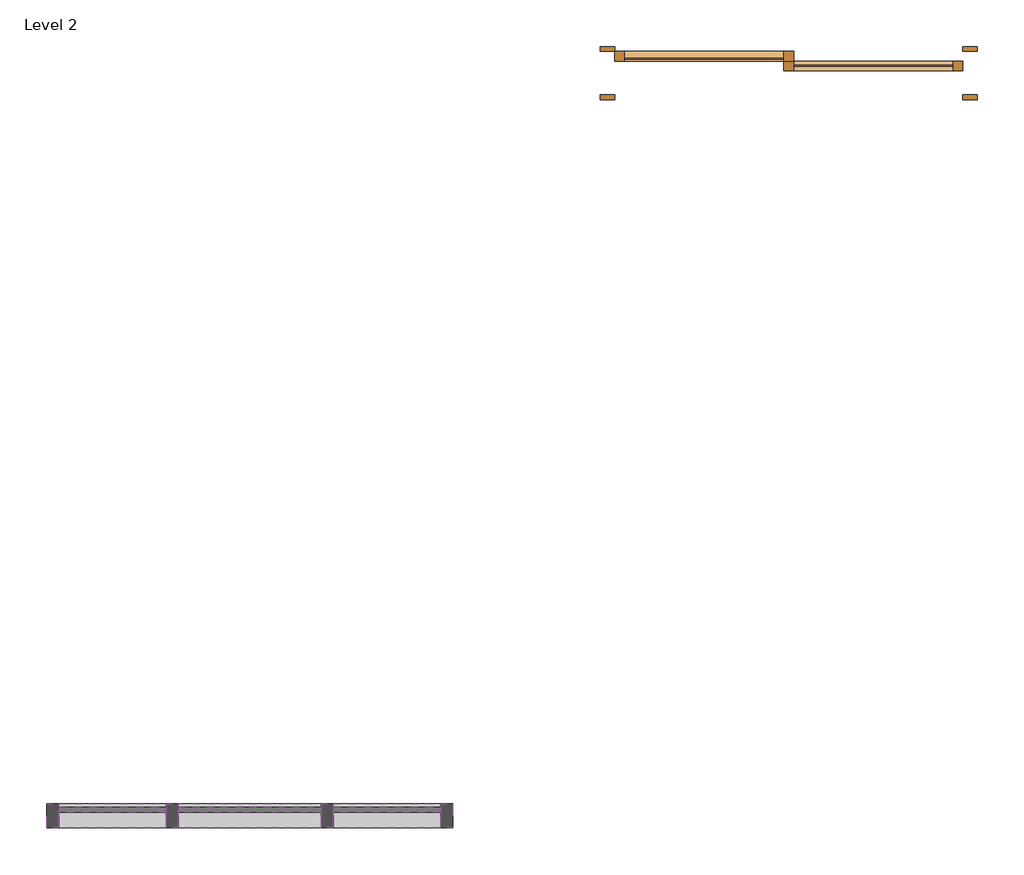
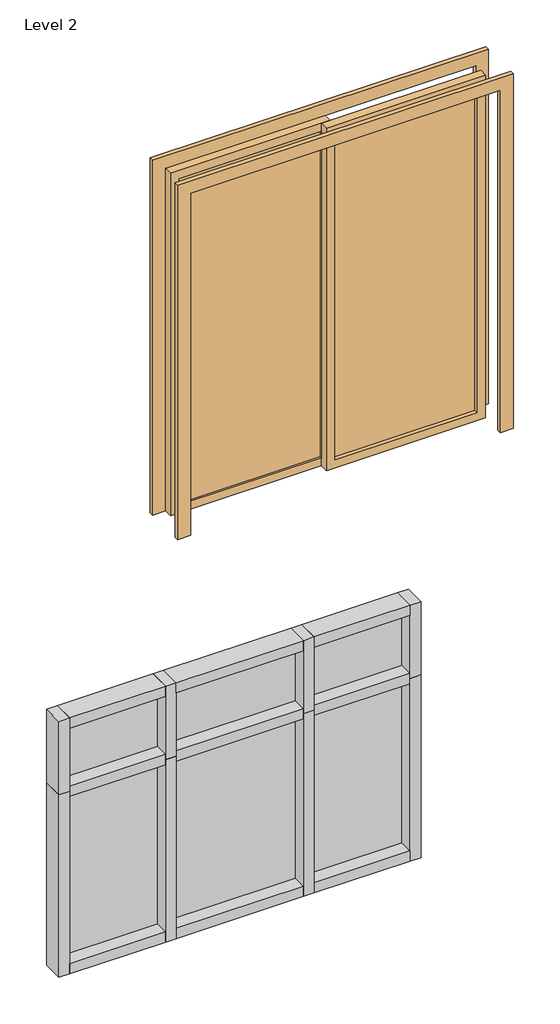
# One storey, incomplete: 17 members, 6 plates, 1 door.
"""IFC4 building model written with IfcOpenShell, lengths in millimetres."""

from ifc_helpers import new_model, si_unit, origin, place, context, project, spatial, transform, mapped, element, save
from components import door_d4d75d1e, member_6f432376, member_9d02be77, member_64b232f9, member_ffd4c858, member_798d6cad, member_6103f85b, member_15823cb3, member_af5dd0cd, system_panel_glazed_8b0ca3bf, system_panel_glazed_ceb8c9d8, system_panel_glazed_0dc12997, system_panel_glazed_336a352b

model = new_model("IFC4")

# Units and contexts
model_context = context("Model", 3, world=origin())
ifc_project = project(units=[si_unit("LENGTHUNIT", "METRE", prefix="MILLI")], contexts=[model_context])

# Site, building, storey
site = spatial("IfcSite", under=ifc_project)
building = spatial("IfcBuilding", under=site)
storey = spatial("IfcBuildingStorey", under=building, Name="Level 2", Elevation=3048.0)

# Door
placement = place(None, origin())
door_shape = door_d4d75d1e(model_context)
element("IfcDoor", 1, ObjectType="Door-Double-Sliding : 72\" x 84\"", at=placement, inside=storey, context=model_context, shape_type="MappedRepresentation", body=[
    mapped(door_shape, transform((-8653.5625709, 4627.4176199, 3048.0), x_axis=(1.0, 0.0, 0.0), y_axis=(0.0, 1.0, 0.0), z_axis=(0.0, 0.0, 1.0))),
])

# Members
member_shape = member_6f432376(model_context)
element("IfcMember", 2, ObjectType="Rectangular Mullion : 2.5\" x 5\" rectangular", at=placement, inside=storey, context=model_context, shape_type="MappedRepresentation", body=[
    mapped(member_shape, transform((-10480.9953834, 854.4262137, 5252.1648635), x_axis=(0.0, 0.0, 1.0), y_axis=(0.0, -1.0, 0.0), z_axis=(1.0, 0.0, 0.0))),
])
element("IfcMember", 3, ObjectType="Rectangular Mullion : 2.5\" x 5\" rectangular", at=placement, inside=storey, context=model_context, shape_type="MappedRepresentation", body=[
    mapped(member_shape, transform((-11922.4453834, 854.4262137, 5252.1648635), x_axis=(0.0, 0.0, 1.0), y_axis=(0.0, -1.0, 0.0), z_axis=(1.0, 0.0, 0.0))),
])
element("IfcMember", 4, ObjectType="Rectangular Mullion : 2.5\" x 5\" rectangular", at=placement, inside=storey, context=model_context, shape_type="MappedRepresentation", body=[
    mapped(member_shape, transform((-12487.5953834, 854.4262137, 3657.6), x_axis=(0.0, 0.0, -1.0), y_axis=(0.0, -1.0, 0.0), z_axis=(-1.0, 0.0, 0.0))),
])
element("IfcMember", 5, ObjectType="Rectangular Mullion : 2.5\" x 5\" rectangular", at=placement, inside=storey, context=model_context, shape_type="MappedRepresentation", body=[
    mapped(member_shape, transform((-11046.1453834, 854.4262137, 3657.6), x_axis=(0.0, 0.0, -1.0), y_axis=(0.0, -1.0, 0.0), z_axis=(-1.0, 0.0, 0.0))),
])
member_2_shape = member_9d02be77(model_context)
element("IfcMember", 6, ObjectType="Rectangular Mullion : 2.5\" x 5\" rectangular", at=placement, inside=storey, context=model_context, shape_type="MappedRepresentation", body=[
    mapped(member_2_shape, transform((-11858.9453834, 854.4262137, 3657.6), x_axis=(0.0, 0.0, -1.0), y_axis=(0.0, -1.0, 0.0), z_axis=(-1.0, 0.0, 0.0))),
])
element("IfcMember", 7, ObjectType="Rectangular Mullion : 2.5\" x 5\" rectangular", at=placement, inside=storey, context=model_context, shape_type="MappedRepresentation", body=[
    mapped(member_2_shape, transform((-11109.6453834, 854.4262137, 5252.1648635), x_axis=(0.0, 0.0, 1.0), y_axis=(0.0, -1.0, 0.0), z_axis=(1.0, 0.0, 0.0))),
])
member_3_shape = member_64b232f9(model_context)
element("IfcMember", 8, ObjectType="Rectangular Mullion : 2.5\" x 5\" rectangular", at=placement, inside=storey, context=model_context, shape_type="MappedRepresentation", body=[
    mapped(member_3_shape, transform((-11077.8953834, 854.4262137, 3657.6), x_axis=(1.0, 0.0, 0.0), y_axis=(0.0, -1.0, 0.0), z_axis=(0.0, 0.0, -1.0))),
])
element("IfcMember", 9, ObjectType="Rectangular Mullion : 2.5\" x 5\" rectangular", at=placement, inside=storey, context=model_context, shape_type="MappedRepresentation", body=[
    mapped(member_3_shape, transform((-11890.6953834, 854.4262137, 3657.6), x_axis=(1.0, 0.0, 0.0), y_axis=(0.0, -1.0, 0.0), z_axis=(0.0, 0.0, -1.0))),
])
member_4_shape = member_ffd4c858(model_context)
element("IfcMember", 10, ObjectType="Rectangular Mullion : 2.5\" x 5\" rectangular", at=placement, inside=storey, context=model_context, shape_type="MappedRepresentation", body=[
    mapped(member_4_shape, transform((-11077.8953834, 854.4262137, 4794.9648635), x_axis=(1.0, 0.0, 0.0), y_axis=(0.0, -1.0, 0.0), z_axis=(0.0, 0.0, -1.0))),
])
element("IfcMember", 11, ObjectType="Rectangular Mullion : 2.5\" x 5\" rectangular", at=placement, inside=storey, context=model_context, shape_type="MappedRepresentation", body=[
    mapped(member_4_shape, transform((-11890.6953834, 854.4262137, 4794.9648635), x_axis=(1.0, 0.0, 0.0), y_axis=(0.0, -1.0, 0.0), z_axis=(0.0, 0.0, -1.0))),
])
member_5_shape = member_798d6cad(model_context)
element("IfcMember", 12, ObjectType="Rectangular Mullion : 2.5\" x 5\" rectangular", at=placement, inside=storey, context=model_context, shape_type="MappedRepresentation", body=[
    mapped(member_5_shape, transform((-11109.6453834, 854.4262137, 4794.9648635), x_axis=(0.0, 0.0, 1.0), y_axis=(0.0, -1.0, 0.0), z_axis=(1.0, 0.0, 0.0))),
])
member_6_shape = member_6103f85b(model_context)
element("IfcMember", 13, ObjectType="Rectangular Mullion : 2.5\" x 5\" rectangular", at=placement, inside=storey, context=model_context, shape_type="MappedRepresentation", body=[
    mapped(member_6_shape, transform((-10480.9953834, 854.4262137, 4794.9648635), x_axis=(0.0, 0.0, 1.0), y_axis=(0.0, -1.0, 0.0), z_axis=(1.0, 0.0, 0.0))),
])
element("IfcMember", 14, ObjectType="Rectangular Mullion : 2.5\" x 5\" rectangular", at=placement, inside=storey, context=model_context, shape_type="MappedRepresentation", body=[
    mapped(member_6_shape, transform((-11922.4453834, 854.4262137, 4794.9648635), x_axis=(0.0, 0.0, 1.0), y_axis=(0.0, -1.0, 0.0), z_axis=(1.0, 0.0, 0.0))),
])
member_7_shape = member_15823cb3(model_context)
element("IfcMember", 15, ObjectType="Rectangular Mullion : 2.5\" x 5\" rectangular", at=placement, inside=storey, context=model_context, shape_type="MappedRepresentation", body=[
    mapped(member_7_shape, transform((-12551.0953834, 854.4262137, 5252.1648635), x_axis=(-1.0, 0.0, 0.0), y_axis=(0.0, -1.0, 0.0), z_axis=(0.0, 0.0, 1.0))),
])
member_8_shape = member_af5dd0cd(model_context)
element("IfcMember", 16, ObjectType="Rectangular Mullion : 2.5\" x 5\" rectangular", at=placement, inside=storey, context=model_context, shape_type="MappedRepresentation", body=[
    mapped(member_8_shape, transform((-10417.4953834, 854.4262137, 3657.6), x_axis=(1.0, 0.0, 0.0), y_axis=(0.0, -1.0, 0.0), z_axis=(0.0, 0.0, -1.0))),
])
element("IfcMember", 17, ObjectType="Rectangular Mullion : 2.5\" x 5\" rectangular", at=placement, inside=storey, context=model_context, shape_type="MappedRepresentation", body=[
    mapped(member_7_shape, transform((-10417.4953834, 854.4262137, 4794.9648635), x_axis=(1.0, 0.0, 0.0), y_axis=(0.0, -1.0, 0.0), z_axis=(0.0, 0.0, -1.0))),
])
element("IfcMember", 18, ObjectType="Rectangular Mullion : 2.5\" x 5\" rectangular", at=placement, inside=storey, context=model_context, shape_type="MappedRepresentation", body=[
    mapped(member_8_shape, transform((-12551.0953834, 854.4262137, 4794.9648635), x_axis=(-1.0, 0.0, 0.0), y_axis=(0.0, -1.0, 0.0), z_axis=(0.0, 0.0, 1.0))),
])

# Plates
system_panel_glazed_shape = system_panel_glazed_8b0ca3bf(model_context)
element("IfcPlate", 19, ObjectType="System Panel : Glazed", at=placement, inside=storey, context=model_context, shape_type="MappedRepresentation", body=[
    mapped(system_panel_glazed_shape, transform((-12205.0203834, 854.4262137, 3721.1), x_axis=(1.0, 0.0, 0.0), y_axis=(0.0, 1.0, 0.0), z_axis=(0.0, 0.0, 1.0))),
])
element("IfcPlate", 20, ObjectType="System Panel : Glazed", at=placement, inside=storey, context=model_context, shape_type="MappedRepresentation", body=[
    mapped(system_panel_glazed_shape, transform((-10763.5703834, 854.4262137, 3721.1), x_axis=(1.0, 0.0, 0.0), y_axis=(0.0, 1.0, 0.0), z_axis=(0.0, 0.0, 1.0))),
])
system_panel_glazed_2_shape = system_panel_glazed_ceb8c9d8(model_context)
element("IfcPlate", 21, ObjectType="System Panel : Glazed", at=placement, inside=storey, context=model_context, shape_type="MappedRepresentation", body=[
    mapped(system_panel_glazed_2_shape, transform((-11484.2953834, 854.4262137, 3721.1), x_axis=(1.0, 0.0, 0.0), y_axis=(0.0, 1.0, 0.0), z_axis=(0.0, 0.0, 1.0))),
])
system_panel_glazed_3_shape = system_panel_glazed_0dc12997(model_context)
element("IfcPlate", 22, ObjectType="System Panel : Glazed", at=placement, inside=storey, context=model_context, shape_type="MappedRepresentation", body=[
    mapped(system_panel_glazed_3_shape, transform((-12205.0203834, 854.4262137, 4826.7148635), x_axis=(1.0, 0.0, 0.0), y_axis=(0.0, 1.0, 0.0), z_axis=(0.0, 0.0, 1.0))),
])
element("IfcPlate", 23, ObjectType="System Panel : Glazed", at=placement, inside=storey, context=model_context, shape_type="MappedRepresentation", body=[
    mapped(system_panel_glazed_3_shape, transform((-10763.5703834, 854.4262137, 4826.7148635), x_axis=(1.0, 0.0, 0.0), y_axis=(0.0, 1.0, 0.0), z_axis=(0.0, 0.0, 1.0))),
])
system_panel_glazed_4_shape = system_panel_glazed_336a352b(model_context)
element("IfcPlate", 24, ObjectType="System Panel : Glazed", at=placement, inside=storey, context=model_context, shape_type="MappedRepresentation", body=[
    mapped(system_panel_glazed_4_shape, transform((-11484.2953834, 854.4262137, 4826.7148635), x_axis=(1.0, 0.0, 0.0), y_axis=(0.0, 1.0, 0.0), z_axis=(0.0, 0.0, 1.0))),
])

save(model, "model.ifc")

# Revit data of these elements
# Type "Door-Double-Sliding : 72\" x 84\""
#   Type Mark = "11"
#   Construction Type Id = "opn-d45"
#   Assembly Code = "C1020"
#   Analytic Construction = "Wood frame, double glass door "
#   Thickness = 0' - 2"
#   Thermal Resistance (R) = 1.8150 (h·ft²·°F)/BTU
#   Heat Transfer Coefficient (U) = 0.5510 BTU/(h·ft²·°F)
#   Height = 7' - 0"
#   Rail Width = 0' - 2"
#   Stiles = 0' - 2"
#   Trim Projection Ext = 0' - 1"
#   Trim Projection Int = 0' - 1"
#   Trim Width = 0' - 3"
#   Width = 6' - 0"
#   Define Thermal Properties by = 1
#   Glazing = Glass
#   Panel Material = Wood - Birch - Solid Stained Light Low Gloss
#   Trim Material = Paint - Sienna
#   Visual Light Transmittance = 0
#   Solar Heat Gain Coefficient = 0
#   Function = (empty or 0)
#   Wall Closure = (empty or 0)
# Type "Rectangular Mullion : 2.5\" x 5\" rectangular"
#   built-in parameter 1007304 = 0.416667 (stored number, unit not read)
#   built-in parameter 1007301 = 0.104167 (stored number, unit not read)
#   built-in parameter 1007300 = 0.104167 (stored number, unit not read)
# Type "System Panel : Glazed"
#   Construction Type Id = "GSP4R"
#   Analytic Construction = "1/8 in Pilkington single glazing"
#   Visual Light Transmittance = 0.9
#   Solar Heat Gain Coefficient = 0.86
#   Heat Transfer Coefficient (U) = 1.18115 BTU/(h·ft²·°F)
#   Define Thermal Properties by = 1
# Element 1 (IfcDoor, "Door-Double-Sliding : 72\" x 84\"")
#   Phase Created = New Construction
#   Materials on its faces: "Paint - Sienna", "Wood - Birch - Solid Stained Light Low Gloss", "Glass"
# Elements 2, 3, 4, 5, 6, 7, 8, 9, 10, 11, 12, 13, 14, 15, 16, 17, 18 (IfcMember, "Rectangular Mullion : 2.5\" x 5\" rectangular")
#   Phase Created = New Construction
#   Materials on its faces: "Aluminum"
# Elements 19, 20, 21, 22, 23, 24 (IfcPlate, "System Panel : Glazed")
#   Phase Created = New Construction
#   Materials on its faces: "Glass"
# Materials
#   "Glass": class "Glass", colour RGB 0 128 192, transparency 0.75, Description = "Soda Lime Glass", Cost = 0
#   "Wood - Birch - Solid Stained Light Low Gloss": class "Wood", colour RGB 210 159 95, transparency 0, Cost = 0
#   "Paint - Sienna": colour RGB 118 70 51, transparency 0, Cost = 0
#   "Aluminum": class "Metal", colour RGB 247 247 247, transparency 0, Description = "Aluminum 6061", Cost = 0
